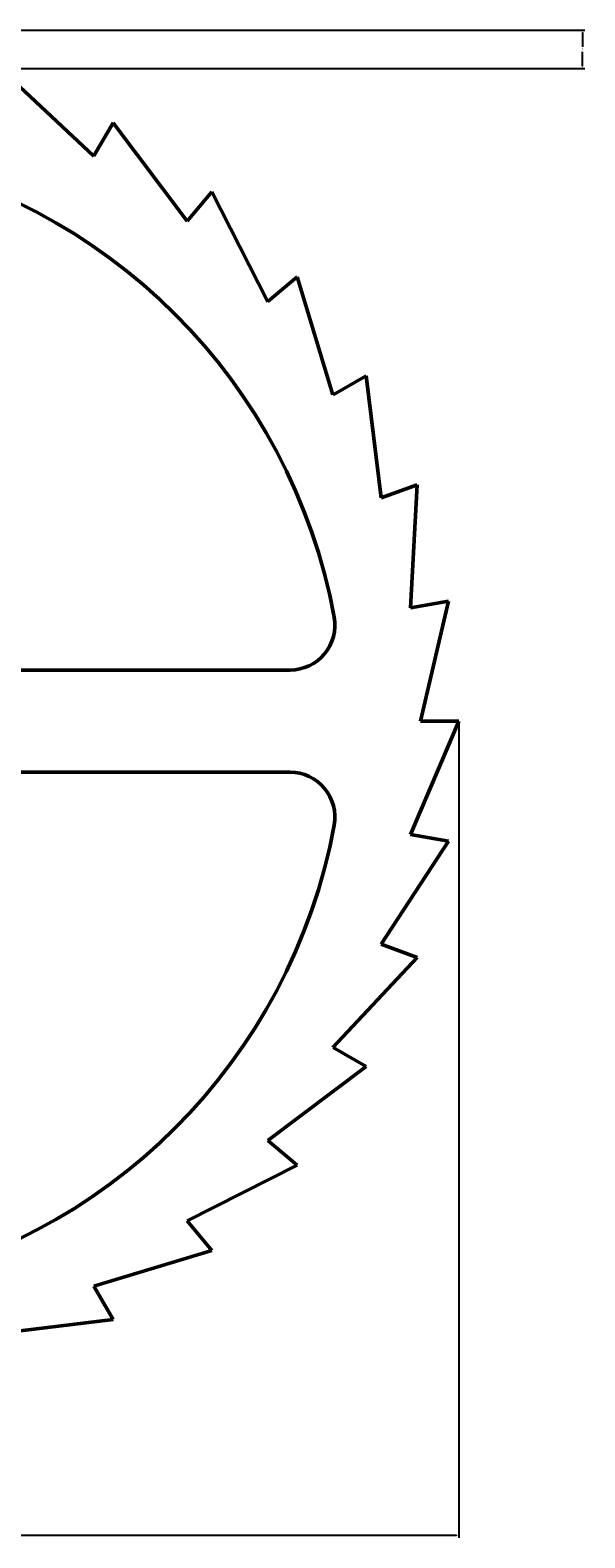
# Model space of a CAD drawing. Units: millimetres. Extents: x 3287 to 3415, y 1573 to 1701.
# Tile 3 of 3: x 3371 to 3415, y 1573 to 1691. Entities that reach past the tile are written whole.
import ezdxf

# ---------------------------------------------------------------- set-up
doc = ezdxf.new("R2010")
doc.units = ezdxf.units.MM
doc.layers.add('M-DIMS', color=2, linetype='Continuous', lineweight=18)
doc.layers.add('M-OUTL', color=7, linetype='Continuous', lineweight=50)
doc.styles.get("Standard").update_dxf_attribs({"font": 'arial.ttf'})
doc.dimstyles.get("Standard").update_dxf_attribs({"dimtxt": 0.18, "dimasz": 0.18, "dimexe": 0.18, "dimexo": 0.0625, "dimgap": 0.09, "dimtad": 0, "dimtih": 1, "dimtoh": 1, "dimdec": 4, "dimzin": 0, "dimdsep": 46, "dimtxsty": 'Standard', "dimcen": 0.09, "dimadec": 0, "dimazin": 0, "dimtfac": 1, "dimtdec": 4, "dimtofl": 0, "dimtmove": 0, "dimatfit": 3, "dimfxl": 1, "dimtolj": 1, "dimtzin": 0, "dimarcsym": 0})

# ---------------------------------------------------------------- blocks, each defined once
blk = doc.blocks.new('RATCHET-TOOTH-10DEG')
for p, q in [((0, 8.86), (2.95, 9.38)), ((2.95, 9.38), (0.77, 0))]:
    blk.add_line(p, q)
blk = doc.blocks.new('WHEEL-SPOKE-OPENING')
for points in [[(40.32, 7.31), (40.32, 36.82)], [(3.5, 0), (33, 0)]]:
    blk.add_lwpolyline(points)
for centre, radius, start, end in [((44.32, -4), 45, 100.4119, 169.5881), ((36.82, 36.82), 3.5, 0, 100.4119), ((3.5, 3.5), 3.5, 169.5881, 270)]:
    blk.add_arc(centre, radius, start, end)
blk = doc.blocks.new('*D3')
at = {"layer": 'Defpoints', "color": 0, "transparency": 16777216}
for p in [(3296.97, 1637.29), (3404.97, 1637.29), (3404.97, 1573.64)]:
    blk.add_point(p, dxfattribs=at)
at = {"layer": 'M-DIMS', "color": 0, "lineweight": -2, "transparency": 16777216}
for p, q in [((3296.97, 1637.22), (3296.97, 1573.46)), ((3404.97, 1637.22), (3404.97, 1573.46)), ((3297.15, 1573.64), (3350.69, 1573.64)), ((3404.79, 1573.64), (3351.25, 1573.64))]:
    blk.add_line(p, q, dxfattribs=at)
at = {"layer": 'M-DIMS', "color": 0, "transparency": 16777216}
for points in [[(3297.15, 1573.67), (3297.15, 1573.61), (3296.97, 1573.64)], [(3404.79, 1573.67), (3404.79, 1573.61), (3404.97, 1573.64)]]:
    blk.add_solid(points, dxfattribs=at)
at = {"layer": 'M-DIMS', "color": 0, "transparency": 16777216, "insert": (3350.97, 1573.64), "char_height": 0.18, "attachment_point": 5}
blk.add_mtext('\\A1;108', dxfattribs=at)
blk = doc.blocks.new('*D5')
at = {"layer": 'Defpoints', "color": 0, "transparency": 16777216}
for p in [(3350.97, 1691.29), (3350.97, 1688.29), (3414.62, 1688.29)]:
    blk.add_point(p, dxfattribs=at)
at = {"layer": 'M-DIMS', "color": 0, "lineweight": -2, "transparency": 16777216}
for p, q in [((3351.03, 1691.29), (3414.8, 1691.29)), ((3414.62, 1691.11), (3414.62, 1689.97)), ((3414.62, 1688.47), (3414.62, 1689.6)), ((3351.03, 1688.29), (3414.8, 1688.29))]:
    blk.add_line(p, q, dxfattribs=at)
at = {"layer": 'M-DIMS', "color": 0, "transparency": 16777216}
for points in [[(3414.59, 1691.11), (3414.65, 1691.11), (3414.62, 1691.29)], [(3414.59, 1688.47), (3414.65, 1688.47), (3414.62, 1688.29)]]:
    blk.add_solid(points, dxfattribs=at)
at = {"layer": 'M-DIMS', "color": 0, "transparency": 16777216, "insert": (3414.62, 1689.79), "char_height": 0.18, "attachment_point": 5}
blk.add_mtext('\\A1;3', dxfattribs=at)

msp = doc.modelspace()

# ---------------------------------------------------------------- block references
at = {"layer": 'M-OUTL'}
for name, p, rotation in [('RATCHET-TOOTH-10DEG', (3376.08, 1680.78), 60.00000000000543), ('RATCHET-TOOTH-10DEG', (3383.26, 1675.76), 50.00000000000177), ('WHEEL-SPOKE-OPENING', (3354.97, 1681.6), 270.0000000000003), ('RATCHET-TOOTH-10DEG', (3389.45, 1669.57), 39.99999999999621), ('RATCHET-TOOTH-10DEG', (3394.47, 1662.4), 30.00000000000043), ('RATCHET-TOOTH-10DEG', (3398.17, 1654.46), 19.99999999999672), ('RATCHET-TOOTH-10DEG', (3400.43, 1646.01), 10.00000000000093), ('RATCHET-TOOTH-10DEG', (3400.43, 1628.56), 350.0000000000036), ('WHEEL-SPOKE-OPENING', (3395.29, 1633.29), 180), ('RATCHET-TOOTH-10DEG', (3398.17, 1620.11), 339.9999999999985), ('RATCHET-TOOTH-10DEG', (3394.47, 1612.17), 330.0000000000013), ('RATCHET-TOOTH-10DEG', (3389.45, 1605), 319.9999999999993), ('RATCHET-TOOTH-10DEG', (3383.26, 1598.81), 310.000000000005), ('RATCHET-TOOTH-10DEG', (3376.08, 1593.79), 299.9999999999977), ('RATCHET-TOOTH-10DEG', (3368.15, 1590.09), 290.0000000000052)]:
    msp.add_blockref(name, p, dxfattribs=dict(at, rotation=rotation))
msp.add_blockref('RATCHET-TOOTH-10DEG', (3401.2, 1637.29), dxfattribs=at)

# ---------------------------------------------------------------- dimensions: what is measured, and where the dimension line sits
at = {"layer": 'M-DIMS'}
dim = msp.add_linear_dim(base=(3414.62, 1688.29), p1=(3350.97, 1691.29), p2=(3350.97, 1688.29), angle=90, dimstyle='Standard', override={"dimdec": 0, "dimlfac": 1, "dimrnd": 0, "dimzin": 0, "dimdsep": 46, "dimlunit": 2}, dxfattribs=at)
dim.commit()
dim.dimension.update_dxf_attribs({"geometry": '*D5', "text_midpoint": (3414.62, 1689.79)})
dim = msp.add_linear_dim(base=(3404.97, 1573.64), p1=(3296.97, 1637.29), p2=(3404.97, 1637.29), dimstyle='Standard', override={"dimdec": 0, "dimlfac": 1, "dimrnd": 0, "dimzin": 0, "dimdsep": 46, "dimlunit": 2}, dxfattribs=at)
dim.commit()
dim.dimension.update_dxf_attribs({"geometry": '*D3', "text_midpoint": (3350.97, 1573.64)})

doc.saveas('drawing.dxf')
